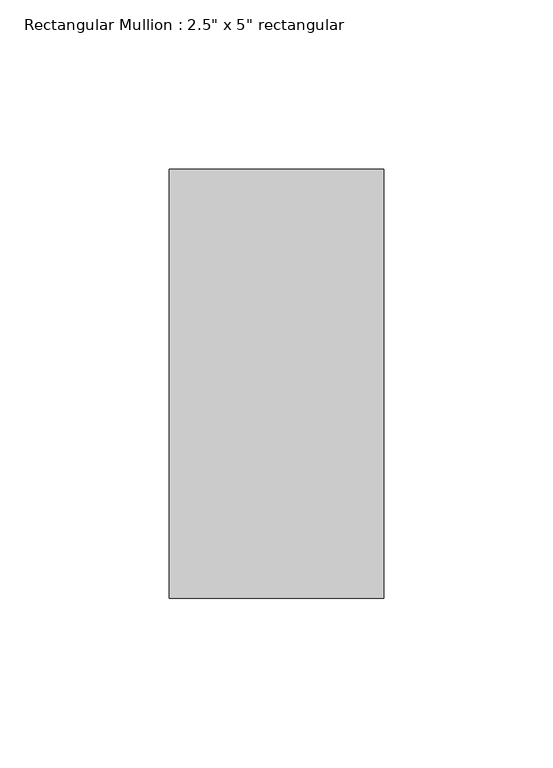
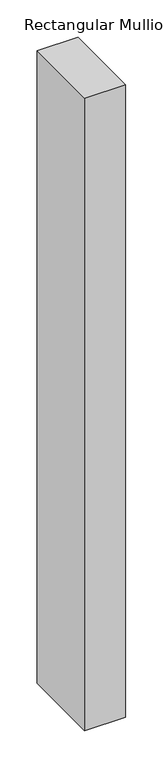
"""IFC4 building model written with IfcOpenShell, lengths in millimetres: member geometry."""

from ifc_helpers import new_model, si_unit, frame, origin, place, context, project, spatial, polyline, outline, extrude, source, transform, mapped, element, save


def member_556b160f(model_context):
    return source(origin(), model_context, "Body", "SweptSolid", [
        extrude(outline(polyline([(31.75, 63.5), (31.75, -63.5), (-31.75, -63.5), (-31.75, 63.5), (31.75, 63.5)])), frame((0.0, 0.0, -1032.9333333), z_axis=(0.0, 0.0, 1.0), x_axis=(1.0, 0.0, 0.0)), (0.0, 0.0, 1.0), 1032.9333333),
    ])


if __name__ == "__main__":
    model = new_model("IFC4")
    model_context = context("Model", 3, world=origin())
    ifc_project = project(units=[si_unit("LENGTHUNIT", "METRE", prefix="MILLI")], contexts=[model_context])
    site = spatial("IfcSite", under=ifc_project)
    building = spatial("IfcBuilding", under=site)
    placement = place(None, origin())
    member_shape = member_556b160f(model_context)
    element("IfcMember", 1, ObjectType="Rectangular Mullion : 2.5\" x 5\" rectangular", at=placement, inside=building, context=model_context, shape_type="MappedRepresentation", body=[
        mapped(member_shape, transform((0.0, 0.0, 0.0), x_axis=(1.0, 0.0, 0.0), y_axis=(0.0, 1.0, 0.0), z_axis=(0.0, 0.0, 1.0))),
    ])
    save(model, "model.ifc")

# Revit data of these elements
# Type "Rectangular Mullion : 2.5\" x 5\" rectangular"
#   built-in parameter 1007304 = 0.416667 (stored number, unit not read)
#   built-in parameter 1007301 = 0.104167 (stored number, unit not read)
#   built-in parameter 1007300 = 0.104167 (stored number, unit not read)
# Element 1 (IfcMember, "Rectangular Mullion : 2.5\" x 5\" rectangular")
#   Materials on its faces: "Aluminum"
# Materials
#   "Aluminum": class "Metal", colour RGB 247 247 247, transparency 0, Description = "Aluminum 6061", Cost = 0
